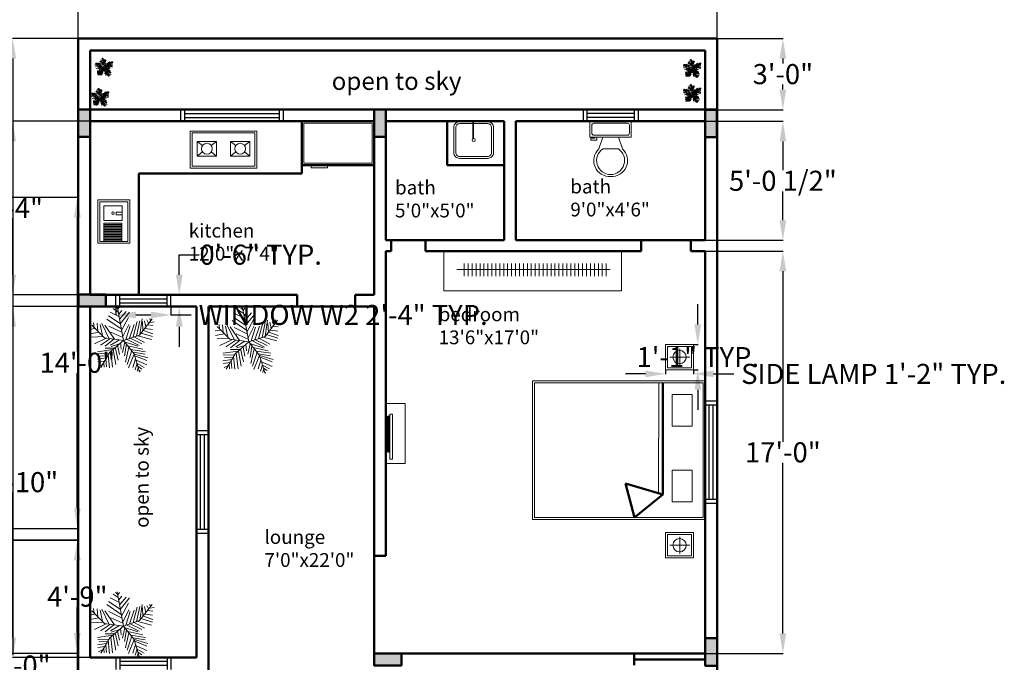
# Model space of a CAD drawing. Units: inches. Extents: x 41 to 5965, y 7 to 3328.
# Tile 3 of 6: x 5442 to 5941, y 2098 to 2424. Entities that reach past the tile are written whole.
import ezdxf

# ---------------------------------------------------------------- set-up
doc = ezdxf.new("R2010")
doc.units = ezdxf.units.IN
doc.header["$MEASUREMENT"] = 0
for name, color, linetype, lineweight in [('A-ANNO-DIMS', 2, 'Continuous', 18), ('A-AREA-IDEN', 3, 'Continuous', 18), ('A-FLOR-FIXT', 9, 'Continuous', 18), ('A-FURN', 8, 'Continuous', 18), ('A-GLAZ', 4, 'Continuous', 25), ('A-WALL', 7, 'Continuous', 50), ('A-WALL-PATT', 8, 'Continuous', 13), ('L-PLNT', 82, 'Continuous', 13)]:
    doc.layers.add(name, color=color, linetype=linetype, lineweight=lineweight)
doc.styles.get("Standard").update_dxf_attribs({"font": 'arial.ttf'})
doc.dimstyles.get("Standard").update_dxf_attribs({"dimtxt": 10.18, "dimasz": 10.18, "dimexe": 0.18, "dimexo": 0.0625, "dimgap": 0.09, "dimtad": 0, "dimtih": 1, "dimtoh": 1, "dimdec": 0, "dimzin": 0, "dimdsep": 46, "dimlunit": 3, "dimtxsty": 'Standard', "dimcen": 0.09, "dimadec": 0, "dimazin": 0, "dimtfac": 1, "dimtdec": 0, "dimtofl": 0, "dimtmove": 0, "dimatfit": 3, "dimfxl": 1, "dimtolj": 1, "dimtzin": 0, "dimarcsym": 0})

# ---------------------------------------------------------------- blocks, each defined once
blk = doc.blocks.new('*U6')
for p, q in [((9.5, -6), (9.5, -2)), ((-10, -8.5), (-8, -8.5)), ((-10, -9.5), (-10, -8.5)), ((-7, -9.5), (-10, -9.5)), ((-8, -8.5), (-8, -8)), ((-7, -8), (-7, -9.5)), ((-4, -8), (-6, -14)), ((4, -8), (6, -14)), ((4, -14), (-4, -14))]:
    blk.add_line(p, q)
blk.add_lwpolyline([(10.5, -8), (10.5, 0), (-10.5, 0), (-10.5, -8)], close=True)
for points in [[(-9.5, -2), (-9.5, -6)], [(8.5, -1), (-8.5, -1)], [(-8.5, -7), (8.5, -7)]]:
    blk.add_lwpolyline(points)
for centre, radius, start, end in [((-8.625, -1.875), 0.8839, 81.8699, 188.1301), ((8.625, -1.875), 0.8839, 351.8699, 98.1301), ((-8.625, -6.125), 0.8839, 171.869898, 278.1301), ((8.625, -6.125), 0.8839, 261.8699, 8.1301), ((-0.4772, -19.9188), 8.0953, 133.01722, 273.38), ((0.0374, -19.8731), 7.127, 124.50543, 269.7), ((-0.0373, -19.8731), 7.127, 270.3, 55.4946), ((0.4773, -19.9188), 8.0953, 266.62, 46.9828)]:
    blk.add_arc(centre, radius, start, end)
blk = doc.blocks.new('*U8')
for p, q in [((-8.737, 47.138), (-17.069, 52.711)), ((-10.186, 53.64), (-13.084, 55.962)), ((0, 0), (-10.5, 57)), ((-9.099, 51.782), (-6.563, 55.962)), ((-7.65, 43.423), (-2.578, 49.46)), ((-3.665, 19.273), (-27.574, 35.527)), ((-5.114, 28.097), (-24.676, 40.636)), ((-7.288, 39.707), (-21.778, 46.673)), ((-5.839, 35.992), (4.667, 48.067)), ((-5.114, 27.632), (10.463, 46.673)), ((-2.941, 16.486), (8.652, 37.85)), ((27, 9), (48, 36)), ((27.127, 9.056), (31.112, 35.992)), ((35.096, 32.741), (37.27, 22.524)), ((38.719, 34.134), (41.979, 28.561)), ((44.153, 36.456), (45.239, 32.741)), ((-47.498, 19.737), (-55.83, 18.344)), ((-31.5, 4.5), (-52.5, 25.5)), ((-48.585, 21.131), (-49.309, 29.026)), ((-43.513, 28.561), (-42.427, 15.558)), ((-38.442, 26.239), (-34.819, 7.663)), ((-35.544, 28.097), (-24.314, 3.947)), ((-14.533, 2.09), (-30.834, 25.31)), ((-24.314, 23.917), (-2.941, 13.7)), ((-1.129, 6.734), (9.014, 26.704)), ((3.942, 1.625), (11.187, 24.381)), ((10.101, 3.483), (17.708, 26.239)), ((16.259, 5.805), (23.142, 31.348)), ((22.055, 7.198), (27.489, 32.277)), ((31.836, 30.883), (32.561, 16.486)), ((33.285, 16.486), (48.862, 10.913)), ((36.183, 19.737), (48.137, 17.88)), ((40.53, 25.775), (48.862, 24.846)), ((43.791, 29.954), (51.036, 30.883)), ((-40.615, 13.7), (-55.105, 10.913)), ((-33.37, 6.269), (-52.207, 5.34)), ((-28.299, 3.483), (-47.86, -5.805)), ((-21.416, 3.018), (-38.079, -8.128)), ((0, 0), (-31.5, 4.5)), ((-15.982, 2.09), (-30.11, -9.521)), ((0, 0), (-22.5, -19.5)), ((-6.563, 1.161), (-21.416, -8.128)), ((-20.691, 13.7), (-1.129, 4.876)), ((0, 0), (27, 9)), ((0, 0), (18, -22.5)), ((6.478, 1.625), (26.04, -8.592)), ((11.187, 3.483), (30.749, -5.805)), ((18.07, 5.805), (35.096, -3.483)), ((24.229, 7.663), (46.688, 1.625)), ((29.662, 12.307), (48.137, 6.269)), ((-17.431, -15.094), (-42.789, -18.809)), ((-15.257, -12.772), (-30.11, -12.772)), ((-6.563, -5.805), (-19.967, -9.985)), ((-17.069, -15.094), (-12.721, -40.172)), ((-13.446, -11.378), (-8.737, -32.741)), ((-9.461, -8.592), (-6.201, -23.453)), ((-4.752, -3.483), (-3.665, -14.629)), ((2.493, -3.019), (-1.491, -20.202)), ((1.769, -2.555), (24.229, -9.521)), ((5.029, -6.27), (2.131, -25.775)), ((9.014, -11.378), (3.58, -35.992)), ((7.565, -9.056), (32.198, -14.629)), ((12.274, -15.094), (36.907, -18.809)), ((-28.299, -29.026), (-42.789, -31.348)), ((-24.314, -21.596), (-42.427, -22.06)), ((-26.849, -26.24), (-40.253, -25.775)), ((-22.5, -19.5), (-37.5, -45)), ((-29.023, -30.884), (-27.936, -43.887)), ((-25.038, -23.918), (-22.865, -45.281)), ((-20.691, -18.345), (-17.793, -44.352)), ((14.085, -16.951), (6.478, -40.172)), ((18.07, -22.524), (8.289, -45.745)), ((20.244, -30.419), (15.897, -44.816)), ((16.259, -19.738), (36.183, -22.989)), ((18, -22.5), (27, -52.5)), ((18.433, -22.524), (40.53, -29.026)), ((19.157, -25.311), (38.719, -33.206)), ((-30.834, -34.135), (-42.427, -35.528)), ((-34.457, -39.708), (-40.978, -42.494)), ((-32.646, -36.921), (-31.921, -44.352)), ((22.78, -37.85), (19.519, -48.532)), ((21.331, -32.741), (39.081, -40.636)), ((22.78, -38.314), (34.372, -44.816)), ((24.591, -45.745), (23.142, -50.854)), ((24.591, -43.423), (30.749, -47.603)), ((26.764, -49.925), (28.213, -50.854))]:
    blk.add_line(p, q)
blk = doc.blocks.new('WIN-1200')
for p, q in [((0, 0), (0, 6)), ((2, 0), (2, 6)), ((50, 0), (50, 6)), ((52, 0), (52, 6)), ((2, 4), (50, 4)), ((2, 2), (50, 2))]:
    blk.add_line(p, q)
blk = doc.blocks.new('WIN-600')
for p, q in [((0, 0), (0, 6)), ((2, 0), (2, 6)), ((26, 0), (26, 6)), ((28, 0), (28, 6)), ((2, 4), (26, 4)), ((2, 2), (26, 2))]:
    blk.add_line(p, q)
blk = doc.blocks.new('LAMP-SIDE')
for p, q in [((7.23, 10.63), (7.23, 1.95)), ((2.17, 6.39), (12.29, 6.39))]:
    blk.add_line(p, q)
for points in [[(0, 12.78), (14.25, 12.78), (14.25, 0), (0, 0)], [(1, 11.78), (13.25, 11.78), (13.25, 1), (1, 1)]]:
    blk.add_lwpolyline(points, close=True)
blk.add_circle((7.12, 6.39), 3.38)
blk = doc.blocks.new('*D22')
at = {"layer": 'A-ANNO-DIMS', "color": 0, "lineweight": -2, "transparency": 16777216}
for p, q in [((5490.49, 2278.46), (5490.49, 2274.14)), ((5518.49, 2278.46), (5518.49, 2274.14)), ((5500.67, 2274.32), (5508.31, 2274.32)), ((5518.49, 2274.32), (5528.67, 2274.32))]:
    blk.add_line(p, q, dxfattribs=at)
at = {"layer": 'A-ANNO-DIMS', "color": 0, "transparency": 16777216}
for points in [[(5500.67, 2276.02), (5500.67, 2272.62), (5490.49, 2274.32)], [(5508.31, 2276.02), (5508.31, 2272.62), (5518.49, 2274.32)]]:
    blk.add_solid(points, dxfattribs=at)
at = {"layer": 'Defpoints', "color": 0, "transparency": 16777216}
for p in [(5490.49, 2278.52), (5518.49, 2278.52), (5518.49, 2274.32)]:
    blk.add_point(p, dxfattribs=at)
at = {"layer": 'A-ANNO-DIMS', "color": 0, "transparency": 16777216, "insert": (5605.82, 2274.32), "char_height": 10.18, "attachment_point": 5}
blk.add_mtext('\\A1;WINDOW W2 2\'-4" TYP.', dxfattribs=at)
blk = doc.blocks.new('*D23')
at = {"layer": 'A-ANNO-DIMS', "color": 0, "lineweight": -2, "transparency": 16777216}
for p, q in [((5522.69, 2294.7), (5522.69, 2304.88)), ((5522.69, 2304.88), (5532.87, 2304.88)), ((5518.56, 2284.52), (5522.87, 2284.52)), ((5518.56, 2278.52), (5522.87, 2278.52)), ((5522.69, 2268.34), (5522.69, 2258.16))]:
    blk.add_line(p, q, dxfattribs=at)
at = {"layer": 'A-ANNO-DIMS', "color": 0, "transparency": 16777216}
for points in [[(5521, 2294.7), (5524.39, 2294.7), (5522.69, 2284.52)], [(5521, 2268.34), (5524.39, 2268.34), (5522.69, 2278.52)]]:
    blk.add_solid(points, dxfattribs=at)
at = {"layer": 'Defpoints', "color": 0, "transparency": 16777216}
for p in [(5518.49, 2284.52), (5522.69, 2284.52), (5518.49, 2278.52)]:
    blk.add_point(p, dxfattribs=at)
at = {"layer": 'A-ANNO-DIMS', "color": 0, "transparency": 16777216, "insert": (5563.99, 2304.88), "char_height": 10.18, "attachment_point": 5}
blk.add_mtext('\\A1;0\'-6" TYP.', dxfattribs=at)
blk = doc.blocks.new('*D24')
at = {"layer": 'A-ANNO-DIMS', "color": 0, "lineweight": -2, "transparency": 16777216}
for p, q in [((5759.15, 2244.42), (5748.97, 2244.42)), ((5769.33, 2246.5), (5769.33, 2244.24)), ((5783.57, 2246.5), (5783.57, 2244.24)), ((5793.75, 2244.42), (5803.93, 2244.42))]:
    blk.add_line(p, q, dxfattribs=at)
at = {"layer": 'A-ANNO-DIMS', "color": 0, "transparency": 16777216}
for points in [[(5759.15, 2246.12), (5759.15, 2242.73), (5769.33, 2244.42)], [(5793.75, 2246.12), (5793.75, 2242.73), (5783.57, 2244.42)]]:
    blk.add_solid(points, dxfattribs=at)
at = {"layer": 'Defpoints', "color": 0, "transparency": 16777216}
for p in [(5769.33, 2246.56), (5783.57, 2246.56), (5783.57, 2244.42)]:
    blk.add_point(p, dxfattribs=at)
at = {"layer": 'A-ANNO-DIMS', "color": 0, "transparency": 16777216, "insert": (5874.94, 2244.42), "char_height": 10.18, "attachment_point": 5}
blk.add_mtext('\\A1;SIDE LAMP 1\'-2" TYP.', dxfattribs=at)
blk = doc.blocks.new('*D25')
at = {"layer": 'A-ANNO-DIMS', "color": 0, "lineweight": -2, "transparency": 16777216}
for p, q in [((5785.71, 2269.52), (5785.71, 2279.7)), ((5783.64, 2259.34), (5785.89, 2259.34)), ((5783.64, 2246.56), (5785.89, 2246.56)), ((5785.71, 2236.38), (5785.71, 2226.2))]:
    blk.add_line(p, q, dxfattribs=at)
at = {"layer": 'A-ANNO-DIMS', "color": 0, "transparency": 16777216}
for points in [[(5784.02, 2269.52), (5787.41, 2269.52), (5785.71, 2259.34)], [(5784.02, 2236.38), (5787.41, 2236.38), (5785.71, 2246.56)]]:
    blk.add_solid(points, dxfattribs=at)
at = {"layer": 'Defpoints', "color": 0, "transparency": 16777216}
for p in [(5783.57, 2259.34), (5785.71, 2259.34), (5783.57, 2246.56)]:
    blk.add_point(p, dxfattribs=at)
at = {"layer": 'A-ANNO-DIMS', "color": 0, "transparency": 16777216, "insert": (5785.71, 2252.95), "char_height": 10.18, "attachment_point": 5}
blk.add_mtext('\\A1;1\'-1" TYP.', dxfattribs=at)
blk = doc.blocks.new('*D41')
at = {"layer": 'A-ANNO-DIMS', "color": 0, "lineweight": -2, "transparency": 16777216}
for p, q in [((5433.48, 2160.2), (5471.17, 2160.2)), ((5470.99, 2150.02), (5470.99, 2002.77)), ((5470.99, 1844.82), (5470.99, 1992.07)), ((5433.55, 1834.64), (5471.17, 1834.64))]:
    blk.add_line(p, q, dxfattribs=at)
at = {"layer": 'A-ANNO-DIMS', "color": 0, "transparency": 16777216}
for points in [[(5469.29, 2150.02), (5472.69, 2150.02), (5470.99, 2160.2)], [(5469.29, 1844.82), (5472.69, 1844.82), (5470.99, 1834.64)]]:
    blk.add_solid(points, dxfattribs=at)
at = {"layer": 'Defpoints', "color": 0, "transparency": 16777216}
for p in [(5433.42, 2160.2), (5470.99, 2160.2), (5433.49, 1834.64)]:
    blk.add_point(p, dxfattribs=at)
at = {"layer": 'A-ANNO-DIMS', "color": 0, "transparency": 16777216, "insert": (5470.99, 1997.42), "char_height": 10.18, "attachment_point": 5}
blk.add_mtext('\\A1;27\'-1 1/2"', dxfattribs=at)
blk = doc.blocks.new('*D42')
at = {"layer": 'A-ANNO-DIMS', "color": 0, "lineweight": -2, "transparency": 16777216}
for p, q in [((5433.36, 2334.08), (5471.17, 2334.08)), ((5470.99, 2323.9), (5470.99, 2255.37)), ((5470.99, 2176.26), (5470.99, 2244.79)), ((5433.36, 2166.08), (5471.17, 2166.08))]:
    blk.add_line(p, q, dxfattribs=at)
at = {"layer": 'A-ANNO-DIMS', "color": 0, "transparency": 16777216}
for points in [[(5469.29, 2323.9), (5472.69, 2323.9), (5470.99, 2334.08)], [(5469.29, 2176.26), (5472.69, 2176.26), (5470.99, 2166.08)]]:
    blk.add_solid(points, dxfattribs=at)
at = {"layer": 'Defpoints', "color": 0, "transparency": 16777216}
for p in [(5433.3, 2334.08), (5470.99, 2334.08), (5433.3, 2166.08)]:
    blk.add_point(p, dxfattribs=at)
at = {"layer": 'A-ANNO-DIMS', "color": 0, "transparency": 16777216, "insert": (5470.99, 2250.08), "char_height": 10.18, "attachment_point": 5}
blk.add_mtext('\\A1;14\'-0"', dxfattribs=at)
blk = doc.blocks.new('*D46')
at = {"layer": 'A-ANNO-DIMS', "color": 0, "lineweight": -2, "transparency": 16777216}
for p, q in [((5365.69, 2160.08), (5471.17, 2160.08)), ((5470.99, 2149.9), (5470.99, 2136.75)), ((5470.99, 2113.02), (5470.99, 2126.17)), ((5365.69, 2102.84), (5471.17, 2102.84))]:
    blk.add_line(p, q, dxfattribs=at)
at = {"layer": 'A-ANNO-DIMS', "color": 0, "transparency": 16777216}
for points in [[(5469.29, 2149.9), (5472.69, 2149.9), (5470.99, 2160.08)], [(5469.29, 2113.02), (5472.69, 2113.02), (5470.99, 2102.84)]]:
    blk.add_solid(points, dxfattribs=at)
at = {"layer": 'Defpoints', "color": 0, "transparency": 16777216}
for p in [(5365.62, 2160.08), (5470.99, 2160.08), (5365.62, 2102.84)]:
    blk.add_point(p, dxfattribs=at)
at = {"layer": 'A-ANNO-DIMS', "color": 0, "transparency": 16777216, "insert": (5470.99, 2131.46), "char_height": 10.18, "attachment_point": 5}
blk.add_mtext('\\A1;4\'-9"', dxfattribs=at)
blk = doc.blocks.new('*D49')
at = {"layer": 'A-ANNO-DIMS', "color": 0, "lineweight": -2, "transparency": 16777216}
for p, q in [((5471.49, 2414.58), (5471.49, 2465.95)), ((5481.67, 2465.77), (5615.83, 2465.77)), ((5785.31, 2465.77), (5651.16, 2465.77)), ((5795.49, 2414.58), (5795.49, 2465.95))]:
    blk.add_line(p, q, dxfattribs=at)
at = {"layer": 'A-ANNO-DIMS', "color": 0, "transparency": 16777216}
for points in [[(5481.67, 2467.47), (5481.67, 2464.07), (5471.49, 2465.77)], [(5785.31, 2467.47), (5785.31, 2464.07), (5795.49, 2465.77)]]:
    blk.add_solid(points, dxfattribs=at)
at = {"layer": 'Defpoints', "color": 0, "transparency": 16777216}
for p in [(5795.49, 2465.77), (5471.49, 2414.52), (5795.49, 2414.52)]:
    blk.add_point(p, dxfattribs=at)
at = {"layer": 'A-ANNO-DIMS', "color": 0, "transparency": 16777216, "insert": (5633.49, 2465.77), "char_height": 10.18, "attachment_point": 5}
blk.add_mtext('\\A1;27\'-0"', dxfattribs=at)
blk = doc.blocks.new('*D50')
at = {"layer": 'A-ANNO-DIMS', "color": 0, "lineweight": -2, "transparency": 16777216}
for p, q in [((5471.43, 2414.52), (5438.06, 2414.52)), ((5438.24, 2404.34), (5438.24, 2101.81)), ((5438.24, 1788.7), (5438.24, 2091.23)), ((5471.43, 1778.52), (5438.06, 1778.52))]:
    blk.add_line(p, q, dxfattribs=at)
at = {"layer": 'A-ANNO-DIMS', "color": 0, "transparency": 16777216}
for points in [[(5436.55, 2404.34), (5439.94, 2404.34), (5438.24, 2414.52)], [(5436.55, 1788.7), (5439.94, 1788.7), (5438.24, 1778.52)]]:
    blk.add_solid(points, dxfattribs=at)
at = {"layer": 'Defpoints', "color": 0, "transparency": 16777216}
for p in [(5438.24, 2414.52), (5471.49, 2414.52), (5471.49, 1778.52)]:
    blk.add_point(p, dxfattribs=at)
at = {"layer": 'A-ANNO-DIMS', "color": 0, "transparency": 16777216, "insert": (5438.24, 2096.52), "char_height": 10.18, "attachment_point": 5}
blk.add_mtext('\\A1;53\'-0"', dxfattribs=at)
blk = doc.blocks.new('*D56')
at = {"layer": 'A-ANNO-DIMS', "color": 0, "lineweight": -2, "transparency": 16777216}
for p, q in [((5789.56, 2306.64), (5829.04, 2306.64)), ((5828.86, 2296.46), (5828.86, 2209.93)), ((5828.86, 2112.82), (5828.86, 2199.35)), ((5789.56, 2102.64), (5829.04, 2102.64))]:
    blk.add_line(p, q, dxfattribs=at)
at = {"layer": 'A-ANNO-DIMS', "color": 0, "transparency": 16777216}
for points in [[(5827.16, 2296.46), (5830.56, 2296.46), (5828.86, 2306.64)], [(5827.16, 2112.82), (5830.56, 2112.82), (5828.86, 2102.64)]]:
    blk.add_solid(points, dxfattribs=at)
at = {"layer": 'Defpoints', "color": 0, "transparency": 16777216}
for p in [(5789.49, 2306.64), (5828.86, 2306.64), (5789.49, 2102.64)]:
    blk.add_point(p, dxfattribs=at)
at = {"layer": 'A-ANNO-DIMS', "color": 0, "transparency": 16777216, "insert": (5828.86, 2204.64), "char_height": 10.18, "attachment_point": 5}
blk.add_mtext('\\A1;17\'-0"', dxfattribs=at)
blk = doc.blocks.new('*D57')
at = {"layer": 'A-ANNO-DIMS', "color": 0, "lineweight": -2, "transparency": 16777216}
for p, q in [((5789.56, 2372.52), (5829.04, 2372.52)), ((5828.86, 2362.34), (5828.86, 2347.71)), ((5828.86, 2322.38), (5828.86, 2337)), ((5789.56, 2312.2), (5829.04, 2312.2))]:
    blk.add_line(p, q, dxfattribs=at)
at = {"layer": 'A-ANNO-DIMS', "color": 0, "transparency": 16777216}
for points in [[(5827.16, 2362.34), (5830.56, 2362.34), (5828.86, 2372.52)], [(5827.16, 2322.38), (5830.56, 2322.38), (5828.86, 2312.2)]]:
    blk.add_solid(points, dxfattribs=at)
at = {"layer": 'Defpoints', "color": 0, "transparency": 16777216}
for p in [(5789.49, 2372.52), (5828.86, 2372.52), (5789.49, 2312.2)]:
    blk.add_point(p, dxfattribs=at)
at = {"layer": 'A-ANNO-DIMS', "color": 0, "transparency": 16777216, "insert": (5828.86, 2342.36), "char_height": 10.18, "attachment_point": 5}
blk.add_mtext('\\A1;5\'-0 1/2"', dxfattribs=at)
blk = doc.blocks.new('*D58')
at = {"layer": 'A-ANNO-DIMS', "color": 0, "lineweight": -2, "transparency": 16777216}
for p, q in [((5795.56, 2414.52), (5829.04, 2414.52)), ((5828.86, 2404.34), (5828.86, 2401.76)), ((5828.86, 2388.59), (5828.86, 2391.17)), ((5789.47, 2378.41), (5829.04, 2378.41))]:
    blk.add_line(p, q, dxfattribs=at)
at = {"layer": 'A-ANNO-DIMS', "color": 0, "transparency": 16777216}
for points in [[(5827.16, 2404.34), (5830.56, 2404.34), (5828.86, 2414.52)], [(5827.16, 2388.59), (5830.56, 2388.59), (5828.86, 2378.41)]]:
    blk.add_solid(points, dxfattribs=at)
at = {"layer": 'Defpoints', "color": 0, "transparency": 16777216}
for p in [(5795.49, 2414.52), (5828.86, 2414.52), (5789.41, 2378.41)]:
    blk.add_point(p, dxfattribs=at)
at = {"layer": 'A-ANNO-DIMS', "color": 0, "transparency": 16777216, "insert": (5828.86, 2396.46), "char_height": 10.18, "attachment_point": 5}
blk.add_mtext('\\A1;3\'-0"', dxfattribs=at)
blk = doc.blocks.new('*D61')
at = {"layer": 'A-ANNO-DIMS', "color": 0, "lineweight": -2, "transparency": 16777216}
for p, q in [((5477.43, 2278.52), (5438.06, 2278.52)), ((5438.24, 2268.34), (5438.24, 2194.81)), ((5438.24, 2110.7), (5438.24, 2184.23)), ((5477.43, 2100.52), (5438.06, 2100.52))]:
    blk.add_line(p, q, dxfattribs=at)
at = {"layer": 'A-ANNO-DIMS', "color": 0, "transparency": 16777216}
for points in [[(5436.55, 2268.34), (5439.94, 2268.34), (5438.24, 2278.52)], [(5436.55, 2110.7), (5439.94, 2110.7), (5438.24, 2100.52)]]:
    blk.add_solid(points, dxfattribs=at)
at = {"layer": 'Defpoints', "color": 0, "transparency": 16777216}
for p in [(5438.24, 2278.52), (5477.49, 2278.52), (5477.49, 2100.52)]:
    blk.add_point(p, dxfattribs=at)
at = {"layer": 'A-ANNO-DIMS', "color": 0, "transparency": 16777216, "insert": (5438.24, 2189.52), "char_height": 10.18, "attachment_point": 5}
blk.add_mtext('\\A1;14\'-10"', dxfattribs=at)
blk = doc.blocks.new('*D62')
at = {"layer": 'A-ANNO-DIMS', "color": 0, "lineweight": -2, "transparency": 16777216}
for p, q in [((5477.43, 2372.52), (5438.06, 2372.52)), ((5438.24, 2362.34), (5438.24, 2333.7)), ((5438.24, 2294.7), (5438.24, 2323.34)), ((5477.43, 2284.52), (5438.06, 2284.52))]:
    blk.add_line(p, q, dxfattribs=at)
at = {"layer": 'A-ANNO-DIMS', "color": 0, "transparency": 16777216}
for points in [[(5436.55, 2362.34), (5439.94, 2362.34), (5438.24, 2372.52)], [(5436.55, 2294.7), (5439.94, 2294.7), (5438.24, 2284.52)]]:
    blk.add_solid(points, dxfattribs=at)
at = {"layer": 'Defpoints', "color": 0, "transparency": 16777216}
for p in [(5438.24, 2372.52), (5477.49, 2372.52), (5477.49, 2284.52)]:
    blk.add_point(p, dxfattribs=at)
at = {"layer": 'A-ANNO-DIMS', "color": 0, "transparency": 16777216, "insert": (5438.24, 2328.52), "char_height": 10.18, "attachment_point": 5}
blk.add_mtext('\\A1;7\'-4"', dxfattribs=at)

msp = doc.modelspace()

# ---------------------------------------------------------------- hatches: boundary and pattern name
at = {"layer": 'A-WALL-PATT'}
h = msp.add_hatch(color=256, dxfattribs=at)
h.dxf.hatch_style = 1
h.paths.add_polyline_path([(5477.49, 2378.52), (5471.49, 2378.52), (5471.49, 2364.59), (5477.49, 2364.59)])
h.paths.add_polyline_path([(5627.49, 2372.52), (5627.52, 2378.52), (5621.52, 2378.52), (5621.52, 2364.59), (5627.49, 2364.59)])
h.paths.add_polyline_path([(5795.41, 2378.41), (5789.41, 2378.41), (5789.41, 2372.52), (5789.49, 2372.52), (5789.49, 2364.48), (5795.41, 2364.48)])
h.paths.add_polyline_path([(5485.48, 2284.52), (5477.49, 2284.52), (5471.55, 2284.61), (5471.55, 2278.61), (5485.48, 2278.61)])
h.paths.add_polyline_path([(5477.49, 2075.53), (5471.54, 2075.53), (5471.54, 2061.6), (5477.49, 2061.6)])
h.paths.add_polyline_path([(5477.49, 1860.52), (5477.49, 1866.7), (5471.52, 1866.7), (5471.52, 1852.76), (5477.49, 1852.76), (5477.49, 1854.52), (5477.51, 1860.52)])
h.paths.add_polyline_path([(5627.43, 1868.54), (5621.49, 1868.54), (5621.49, 1860.52), (5621.43, 1854.61), (5627.43, 1854.61)])
h.paths.add_polyline_path([(5795.49, 1865.02), (5789.61, 1865.02), (5789.61, 1851.08), (5795.49, 1851.08)])
h.paths.add_polyline_path([(5795.48, 2110.36), (5789.49, 2110.36), (5789.49, 2102.64), (5789.49, 2096.43), (5795.48, 2096.43)])
h.paths.add_polyline_path([(5795.4, 2037.71), (5789.49, 2037.71), (5789.49, 2031.57), (5789.49, 2023.78), (5795.4, 2023.78)])
h.paths.add_polyline_path([(5635.41, 2102.54), (5621.49, 2102.54), (5621.49, 2096.64), (5627.49, 2096.64), (5635.41, 2096.64)])

# ---------------------------------------------------------------- linework, layer by layer
at = {"layer": 'A-FLOR-FIXT'}
for p, q in [((5531.83, 2362.33), (5534.54, 2360.27)), ((5541.6, 2362.33), (5538.9, 2360.27)), ((5548.72, 2362.33), (5551.43, 2360.27)), ((5558.5, 2362.33), (5555.79, 2360.27)), ((5531.83, 2354.91), (5534.54, 2356.96)), ((5541.6, 2354.91), (5538.9, 2356.96)), ((5548.72, 2354.91), (5551.43, 2356.96)), ((5558.5, 2354.91), (5555.79, 2356.96))]:
    msp.add_line(p, q, dxfattribs=at)
for points in [[(5661.93, 2369.36, -0.414214), (5664.93, 2372.36), (5679.12, 2372.36, -0.414214), (5682.12, 2369.36), (5682.12, 2356.7, -0.414214), (5679.12, 2353.7), (5664.93, 2353.7, -0.414214), (5661.93, 2356.7)], [(5662.93, 2369.36, -0.414214), (5664.93, 2371.36), (5679.12, 2371.36, -0.414214), (5681.12, 2369.36), (5681.12, 2356.7, -0.414214), (5679.12, 2354.7), (5664.93, 2354.7, -0.414214), (5662.93, 2356.7)]]:
    msp.add_lwpolyline(points, format="xyb", close=True, dxfattribs=at)
for points in [[(5672.02, 2372.36), (5672.02, 2372.36), (5671.54, 2372.36), (5671.54, 2372.36), (5671.54, 2363.65), (5671.54, 2363.65), (5672.02, 2363.65), (5672.02, 2363.65)], [(5528.22, 2367.6), (5562.02, 2367.6), (5562.02, 2348.78), (5528.22, 2348.78)], [(5585.89, 2371.52), (5620.49, 2371.52), (5620.49, 2351.25), (5585.89, 2351.25)], [(5529.22, 2366.6), (5561.02, 2366.6), (5561.02, 2349.78), (5529.22, 2349.78)], [(5531.83, 2362.33), (5541.6, 2362.33), (5541.6, 2354.91), (5531.83, 2354.91)], [(5548.72, 2362.33), (5558.5, 2362.33), (5558.5, 2354.91), (5548.72, 2354.91)], [(5589.59, 2350.25), (5589.59, 2350.25), (5597.84, 2350.25), (5597.84, 2350.25), (5597.84, 2348.99), (5597.84, 2348.99), (5589.59, 2348.99), (5589.59, 2348.99)], [(5481.47, 2332.64), (5497.54, 2332.64), (5497.54, 2310.64), (5481.47, 2310.64)], [(5482.47, 2331.64), (5496.54, 2331.64), (5496.54, 2311.64), (5482.47, 2311.64)], [(5484.5, 2329.63), (5493.66, 2329.63), (5493.66, 2322.21), (5484.5, 2322.21)], [(5493.66, 2326.5), (5490.62, 2326.5), (5490.62, 2325.17), (5493.66, 2325.17)], [(5484.52, 2320.87), (5493.58, 2320.87), (5493.58, 2320.23), (5484.52, 2320.23)], [(5484.52, 2320.23), (5493.58, 2320.23), (5493.58, 2319.59), (5484.52, 2319.59)], [(5484.52, 2319.59), (5493.58, 2319.59), (5493.58, 2318.96), (5484.52, 2318.96)], [(5484.52, 2318.96), (5493.58, 2318.96), (5493.58, 2318.32), (5484.52, 2318.32)], [(5484.52, 2318.32), (5493.58, 2318.32), (5493.58, 2317.68), (5484.52, 2317.68)], [(5484.52, 2317.68), (5493.58, 2317.68), (5493.58, 2317.05), (5484.52, 2317.05)], [(5484.52, 2317.05), (5493.58, 2317.05), (5493.58, 2316.41), (5484.52, 2316.41)], [(5484.52, 2316.41), (5493.58, 2316.41), (5493.58, 2315.77), (5484.52, 2315.77)], [(5484.52, 2315.77), (5493.58, 2315.77), (5493.58, 2315.13), (5484.52, 2315.13)], [(5484.52, 2315.13), (5493.58, 2315.13), (5493.58, 2314.5), (5484.52, 2314.5)], [(5484.52, 2314.5), (5493.58, 2314.5), (5493.58, 2313.86), (5484.52, 2313.86)], [(5484.52, 2313.86), (5493.58, 2313.86), (5493.58, 2313.22), (5484.52, 2313.22)], [(5484.52, 2313.22), (5493.58, 2313.22), (5493.58, 2312.59), (5484.52, 2312.59)], [(5484.52, 2312.59), (5493.58, 2312.59), (5493.58, 2311.95), (5484.52, 2311.95)]]:
    msp.add_lwpolyline(points, close=True, dxfattribs=at)
for centre, radius in [((5672.02, 2363.03), 0.791), ((5536.72, 2358.62), 2.74), ((5553.61, 2358.62), 2.74), ((5489.08, 2325.92), 0.66)]:
    msp.add_circle(centre, radius, dxfattribs=at)
at = {"layer": 'A-FURN'}
for p, q in [((5663.54, 2297.35), (5741.25, 2297.35)), ((5667.26, 2300.45), (5667.26, 2293.91)), ((5669.26, 2300.45), (5669.26, 2293.91)), ((5671.26, 2300.45), (5671.26, 2293.91)), ((5673.26, 2300.45), (5673.26, 2293.91)), ((5675.26, 2300.45), (5675.26, 2293.91)), ((5677.26, 2300.45), (5677.26, 2293.91)), ((5679.26, 2300.45), (5679.26, 2293.91)), ((5681.26, 2300.45), (5681.26, 2293.91)), ((5683.26, 2300.45), (5683.26, 2293.91)), ((5685.26, 2300.45), (5685.26, 2293.91)), ((5687.26, 2300.45), (5687.26, 2293.91)), ((5689.26, 2300.45), (5689.26, 2293.91)), ((5691.26, 2300.45), (5691.26, 2293.91)), ((5693.26, 2300.45), (5693.26, 2293.91)), ((5695.26, 2300.45), (5695.26, 2293.91)), ((5697.26, 2300.45), (5697.26, 2293.91)), ((5699.26, 2300.45), (5699.26, 2293.91)), ((5701.26, 2300.45), (5701.26, 2293.91)), ((5703.26, 2300.45), (5703.26, 2293.91)), ((5705.26, 2300.45), (5705.26, 2293.91)), ((5707.26, 2300.45), (5707.26, 2293.91)), ((5709.26, 2300.45), (5709.26, 2293.91)), ((5711.26, 2300.45), (5711.26, 2293.91)), ((5713.26, 2300.45), (5713.26, 2293.91)), ((5715.26, 2300.45), (5715.26, 2293.91)), ((5717.26, 2300.45), (5717.26, 2293.91)), ((5719.26, 2300.45), (5719.26, 2293.91)), ((5721.26, 2300.45), (5721.26, 2293.91)), ((5723.26, 2300.45), (5723.26, 2293.91)), ((5725.26, 2300.45), (5725.26, 2293.91)), ((5727.26, 2300.45), (5727.26, 2293.91)), ((5729.26, 2300.45), (5729.26, 2293.91)), ((5731.26, 2300.45), (5731.26, 2293.91)), ((5733.26, 2300.45), (5733.26, 2293.91)), ((5735.26, 2300.45), (5735.26, 2293.91)), ((5737.26, 2300.45), (5737.26, 2293.91)), ((5739.26, 2300.45), (5739.26, 2293.91)), ((5765.89, 2239.92), (5765.84, 2183.95))]:
    msp.add_line(p, q, dxfattribs=at)
for points in [[(5656.97, 2306.64), (5746.97, 2306.64), (5746.97, 2286.51), (5656.97, 2286.51)], [(5789.49, 2240.92), (5701.87, 2240.92), (5701.87, 2170.55), (5789.49, 2170.55)], [(5788.49, 2239.92), (5702.87, 2239.92), (5702.87, 2171.55), (5788.49, 2171.55)], [(5772.73, 2234), (5782.77, 2234), (5782.77, 2217.95), (5772.73, 2217.95)], [(5627.49, 2229.38), (5637.33, 2229.38), (5637.33, 2199.04), (5627.49, 2199.04)], [(5630.84, 2224.04), (5629.57, 2224.04), (5629.57, 2201.15), (5630.84, 2201.15)], [(5772.73, 2195.56), (5782.77, 2195.56), (5782.77, 2179.5), (5772.73, 2179.5)]]:
    msp.add_lwpolyline(points, close=True, dxfattribs=at)
at = {"layer": 'A-WALL'}
for p, q in [((5471.49, 2378.52), (5471.49, 2414.52)), ((5471.49, 2414.52), (5795.49, 2414.52)), ((5795.49, 2414.52), (5795.49, 2378.52)), ((5477.49, 2408.52), (5789.49, 2408.52)), ((5477.49, 2378.52), (5477.49, 2408.52)), ((5789.49, 2408.52), (5789.49, 2378.52)), ((5471.49, 1778.52), (5471.49, 2378.52)), ((5471.49, 2378.52), (5795.49, 2378.52)), ((5795.49, 2378.52), (5795.49, 1778.52)), ((5477.49, 2372.52), (5621.49, 2372.52)), ((5477.49, 2284.52), (5477.49, 2372.52)), ((5584.89, 2345.98), (5584.89, 2372.52)), ((5621.49, 2284.52), (5621.49, 2372.52)), ((5627.49, 2312.2), (5627.49, 2372.52)), ((5627.49, 2372.52), (5687.49, 2372.52)), ((5658.53, 2372.52), (5658.53, 2350.32)), ((5687.49, 2312.2), (5687.49, 2372.52)), ((5687.56, 2372.36), (5687.56, 2350.32)), ((5693.49, 2312.2), (5693.49, 2372.52)), ((5693.49, 2372.52), (5789.49, 2372.52)), ((5789.49, 2372.52), (5789.49, 2312.2)), ((5687.56, 2350.32), (5658.53, 2350.32)), ((5502.14, 2284.52), (5502.14, 2345.98)), ((5502.14, 2345.98), (5584.89, 2345.98)), ((5627.49, 2312.2), (5687.49, 2312.2)), ((5630.22, 2312.2), (5630.22, 2306.64)), ((5647.61, 2312.2), (5647.61, 2306.64)), ((5693.49, 2312.2), (5789.49, 2312.2)), ((5757.06, 2312.2), (5757.06, 2306.64)), ((5782.21, 2312.2), (5782.21, 2306.64)), ((5627.49, 2152.12), (5627.49, 2306.64)), ((5627.49, 2306.64), (5630.22, 2306.64)), ((5647.61, 2306.64), (5757.06, 2306.64)), ((5687.49, 2306.52), (5687.49, 2306.64)), ((5693.49, 2306.52), (5693.49, 2306.64)), ((5782.21, 2306.64), (5789.49, 2306.64)), ((5789.49, 2306.64), (5789.49, 2102.64)), ((5477.49, 2284.52), (5582.48, 2284.52)), ((5582.48, 2284.52), (5582.48, 2278.52)), ((5612, 2284.52), (5612, 2278.52)), ((5612, 2284.52), (5621.49, 2284.52)), ((5477.49, 2278.52), (5531.49, 2278.52)), ((5477.49, 2100.52), (5477.49, 2278.52)), ((5531.49, 2278.52), (5531.49, 2100.52)), ((5537.49, 2278.52), (5537.49, 2010.52)), ((5537.49, 2278.52), (5621.49, 2278.52)), ((5621.49, 2278.52), (5621.49, 2096.64)), ((5767.99, 2239.92), (5767.99, 2183.33)), ((5629.57, 2222.55), (5628.62, 2223)), ((5628.62, 2223), (5628.62, 2204.7)), ((5628.62, 2204.7), (5629.57, 2205.77)), ((5753.56, 2171.55), (5749.04, 2188.83)), ((5749.04, 2188.83), (5767.99, 2183.33)), ((5767.99, 2183.33), (5753.56, 2171.55)), ((5627.49, 2152.12), (5621.49, 2152.12)), ((5627.49, 2102.64), (5621.49, 2102.64)), ((5627.49, 2102.64), (5789.49, 2102.64)), ((5753.49, 2096.64), (5753.49, 2102.64)), ((5789.49, 2102.64), (5789.49, 2096.64)), ((5477.49, 2100.52), (5531.49, 2100.52)), ((5753.49, 2099.64), (5789.49, 2099.64))]:
    msp.add_line(p, q, dxfattribs=at)
for points in [[(5471.49, 2378.52), (5477.49, 2378.52), (5477.49, 2364.59), (5471.49, 2364.59)], [(5621.52, 2378.53), (5627.52, 2378.53), (5627.52, 2364.59), (5621.52, 2364.59)], [(5789.41, 2378.41), (5795.41, 2378.41), (5795.41, 2364.48), (5789.41, 2364.48)], [(5584.89, 2372.52), (5584.89, 2372.52), (5621.49, 2372.52), (5621.49, 2372.52), (5621.49, 2350.25), (5621.49, 2350.25), (5584.89, 2350.25), (5584.89, 2350.25)], [(5485.48, 2284.61), (5485.48, 2278.61), (5471.55, 2278.61), (5471.55, 2284.61)], [(5789.48, 2110.36), (5795.48, 2110.36), (5795.48, 2096.43), (5789.48, 2096.43)], [(5635.41, 2102.54), (5635.41, 2096.54), (5621.48, 2096.54), (5621.48, 2102.54)]]:
    msp.add_lwpolyline(points, close=True, dxfattribs=at)

# ---------------------------------------------------------------- block references
at = {"layer": 'A-FLOR-FIXT'}
msp.add_blockref('*U6', (5741.49, 2372.52), dxfattribs=at)
at = {"layer": 'A-FURN'}
for p in [(5769.33, 2246.56), (5769.33, 2151.13)]:
    msp.add_blockref('LAMP-SIDE', p, dxfattribs=at)
at = {"layer": 'A-GLAZ'}
for name, p in [('WIN-1200', (5523.49, 2372.52)), ('WIN-600', (5490.49, 2278.52))]:
    msp.add_blockref(name, p, dxfattribs=at)
for name, p, rotation in [('WIN-600', (5755.49, 2378.52), 180), ('WIN-1200', (5795.49, 2178.64), 89.99999999999616), ('WIN-1200', (5537.49, 2163.52), 89.99999999999186), ('WIN-600', (5518.49, 2100.52), 180)]:
    msp.add_blockref(name, p, dxfattribs=dict(at, rotation=rotation))
at = {"layer": 'L-PLNT'}
for p, xscale, yscale, zscale in [((5484.71, 2399.76), 0.0860075486317361, 0.0860075486317361, 0.0860075486317361), ((5783.05, 2399.09), 0.0860075486317361, 0.0860075486317361, 0.0860075486317361), ((5482.71, 2384.51), 0.0860075486317361, 0.0860075486317361, 0.0860075486317361), ((5783.05, 2386.43), 0.0860075486317361, 0.0860075486317361, 0.0860075486317361), ((5494.34, 2261.39), 0.3056693623898039, 0.3056693623898039, 0.3056693623898039), ((5557.93, 2260.62), 0.3056693623898039, 0.3056693623898039, 0.3056693623898039), ((5494.34, 2116.52), 0.3056693623898039, 0.3056693623898039, 0.3056693623898039)]:
    msp.add_blockref('*U8', p, dxfattribs=dict(at, xscale=xscale, yscale=yscale, zscale=zscale))

# ---------------------------------------------------------------- texts
at = {"layer": 'A-AREA-IDEN', "attachment_point": 1}
for s, width, insert, char_height in [('open to sky', 81.7364, (5600.01, 2397.45), 9), ('bath\\P5\'0"x5\'0"', 52.5564, (5632.14, 2342.45), 7), ('bath\\P9\'0"x4\'6"', 52.5564, (5721.05, 2342.95), 7), ('kitchen\\P12\'0"x7\'4"', 52.5564, (5527.51, 2320.57), 7), ('bedroom\\P13\'6"x17\'0"', 52.5564, (5654.26, 2278.13), 7), ('lounge\\P7\'0"x22\'0"', 52.5564, (5565.9, 2165.19), 7)]:
    msp.add_mtext_dynamic_manual_height_columns(s, width=width, gutter_width=1, heights=[0], dxfattribs=dict(at, insert=insert, char_height=char_height))
at = {"layer": 'A-AREA-IDEN', "insert": (5500.17, 2166.33), "char_height": 7, "attachment_point": 1, "rotation": 90}
msp.add_mtext_dynamic_manual_height_columns('open to sky', width=52.5564, gutter_width=1, heights=[0], dxfattribs=at)

# ---------------------------------------------------------------- dimensions: what is measured, and where the dimension line sits
at = {"layer": 'A-ANNO-DIMS'}
dim = msp.add_linear_dim(base=(5795.49, 2465.77), p1=(5471.49, 2414.52), p2=(5795.49, 2414.52), dimstyle='Standard', override={"dimdec": 1, "dimlfac": 1, "dimrnd": 0, "dimzin": 1, "dimdsep": 46, "dimlunit": 4, "dimfrac": 2}, dxfattribs=at)
dim.commit()
dim.dimension.update_dxf_attribs({"geometry": '*D49', "text_midpoint": (5633.49, 2465.77)})
for base, p1, p2, picture, middle in [((5438.24, 2414.52), (5471.49, 1778.52), (5471.49, 2414.52), '*D50', (5438.24, 2096.52)), ((5828.86, 2414.52), (5789.41, 2378.41), (5795.49, 2414.52), '*D58', (5828.86, 2396.46)), ((5438.24, 2372.52), (5477.49, 2284.52), (5477.49, 2372.52), '*D62', (5438.24, 2328.52)), ((5828.86, 2372.52), (5789.49, 2312.2), (5789.49, 2372.52), '*D57', (5828.86, 2342.36)), ((5470.99, 2334.08), (5433.3, 2166.08), (5433.3, 2334.08), '*D42', (5470.99, 2250.08)), ((5828.86, 2306.64), (5789.49, 2102.64), (5789.49, 2306.64), '*D56', (5828.86, 2204.64)), ((5438.24, 2278.52), (5477.49, 2100.52), (5477.49, 2278.52), '*D61', (5438.24, 2189.52)), ((5470.99, 2160.08), (5365.62, 2102.84), (5365.62, 2160.08), '*D46', (5470.99, 2131.46)), ((5470.99, 2160.2), (5433.49, 1834.64), (5433.42, 2160.2), '*D41', (5470.99, 1997.42))]:
    dim = msp.add_linear_dim(base=base, p1=p1, p2=p2, angle=90, dimstyle='Standard', override={"dimdec": 1, "dimlfac": 1, "dimrnd": 0, "dimzin": 1, "dimdsep": 46, "dimlunit": 4, "dimfrac": 2}, dxfattribs=at)
    dim.commit()
    dim.dimension.update_dxf_attribs({"geometry": picture, "text_midpoint": middle})
for base, p1, p2, picture, middle in [((5522.69, 2284.52), (5518.49, 2278.52), (5518.49, 2284.52), '*D23', (5563.99, 2304.88)), ((5785.71, 2259.34), (5783.57, 2246.56), (5783.57, 2259.34), '*D25', (5785.71, 2252.95))]:
    dim = msp.add_linear_dim(base=base, p1=p1, p2=p2, angle=90, text='<> TYP.', dimstyle='Standard', override={"dimdec": 1, "dimrnd": 0, "dimzin": 1, "dimlunit": 4, "dimfrac": 2}, dxfattribs=at)
    dim.commit()
    dim.dimension.update_dxf_attribs({"geometry": picture, "text_midpoint": middle})
for base, p1, p2, text, picture, middle in [((5518.49, 2274.32), (5490.49, 2278.52), (5518.49, 2278.52), 'WINDOW W2 <> TYP.', '*D22', (5605.82, 2274.32)), ((5783.57, 2244.42), (5769.33, 2246.56), (5783.57, 2246.56), 'SIDE LAMP <> TYP.', '*D24', (5874.94, 2244.42))]:
    dim = msp.add_linear_dim(base=base, p1=p1, p2=p2, text=text, dimstyle='Standard', override={"dimdec": 1, "dimrnd": 0, "dimzin": 1, "dimlunit": 4, "dimfrac": 2}, dxfattribs=at)
    dim.commit()
    dim.dimension.update_dxf_attribs({"geometry": picture, "text_midpoint": middle})

doc.saveas('drawing.dxf')
